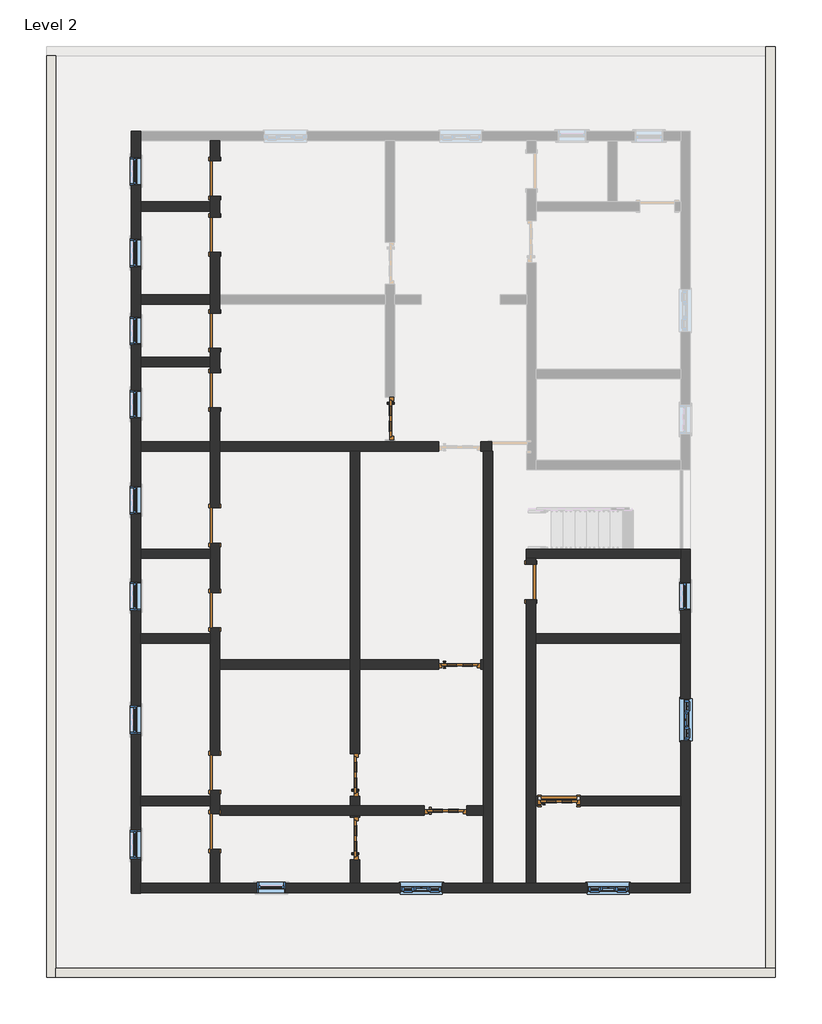
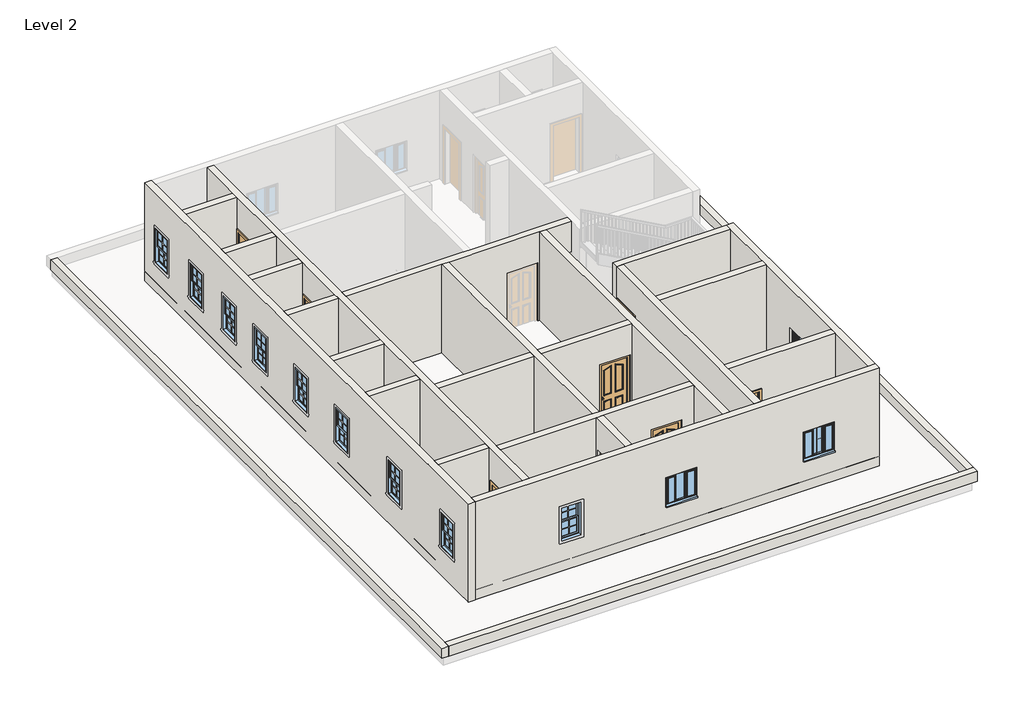
# One storey, part 1 of 3: 22 walls, 16 doors, 13 windows.
# Revit data of these elements (continued)
# Element 44 (IfcWindow, "Window-Double-Hung : 24\" x 42\"")
#   Mark = "28"
#   Window Inset = 0' - 0"
#   Interior Wall Closure = 0' - 1 1/2"
#   Frame Extension = 0' - 1 1/4"
#   Exterior Wall Closure = 0' - 0 1/2"
#   Interior Trim Visibility = yes
#   Indicator Visibility = yes
#   Exterior Trim Visibility = yes
#   Phase Created = New Construction
#   Materials on its faces: "Wood - Stained", "Glass", "Clad - White"
# Element 45 (IfcWindow, "Window-Double-Hung : 24\" x 42\"")
#   Mark = "29"
#   Window Inset = 0' - 0"
#   Interior Wall Closure = 0' - 1 1/2"
#   Frame Extension = 0' - 1 1/4"
#   Exterior Wall Closure = 0' - 0 1/2"
#   Interior Trim Visibility = yes
#   Indicator Visibility = yes
#   Exterior Trim Visibility = yes
#   Phase Created = New Construction
#   Materials on its faces: "Wood - Stained", "Glass", "Clad - White"
# Element 46 (IfcWindow, "Window-Double-Hung : 24\" x 42\"")
#   Mark = "30"
#   Window Inset = 0' - 0"
#   Interior Wall Closure = 0' - 1 1/2"
#   Frame Extension = 0' - 1 1/4"
#   Exterior Wall Closure = 0' - 0 1/2"
#   Interior Trim Visibility = yes
#   Indicator Visibility = yes
#   Exterior Trim Visibility = yes
#   Phase Created = New Construction
#   Materials on its faces: "Wood - Stained", "Glass", "Clad - White"
# Element 47 (IfcWindow, "Window-Double-Hung : 24\" x 42\"")
#   Mark = "31"
#   Window Inset = 0' - 0"
#   Interior Wall Closure = 0' - 1 1/2"
#   Frame Extension = 0' - 1 1/4"
#   Exterior Wall Closure = 0' - 0 1/2"
#   Interior Trim Visibility = yes
#   Indicator Visibility = yes
#   Exterior Trim Visibility = yes
#   Phase Created = New Construction
#   Materials on its faces: "Wood - Stained", "Glass", "Clad - White"
# Element 48 (IfcWindow, "Window-Double-Hung : 24\" x 42\"")
#   Mark = "32"
#   Window Inset = 0' - 0"
#   Interior Wall Closure = 0' - 1 1/2"
#   Frame Extension = 0' - 1 1/4"
#   Exterior Wall Closure = 0' - 0 1/2"
#   Interior Trim Visibility = yes
#   Indicator Visibility = yes
#   Exterior Trim Visibility = yes
#   Phase Created = New Construction
#   Materials on its faces: "Wood - Stained", "Glass", "Clad - White"
# Element 49 (IfcWindow, "Windows_Tpl_w-Glazing_Cross-Bars : 910x910mm")
#   Mark = "20"
#   Phase Created = New Construction
#   Materials on its faces: "Window Frame", "Glass"
# Element 50 (IfcWindow, "Windows_Tpl_w-Glazing_Cross-Bars : 910x910mm")
#   Mark = "37"
#   Phase Created = New Construction
#   Materials on its faces: "Window Frame", "Glass"
# Element 51 (IfcWindow, "Windows_Tpl_w-Glazing_Cross-Bars : 910x910mm")
#   Mark = "38"
#   Phase Created = New Construction
#   Materials on its faces: "Window Frame", "Glass"
# Materials
#   "Door - Glazing": colour RGB 0 0 255, transparency 0.75
#   "Door - Panel": class "Wood", colour RGB 210 159 95, transparency 0, Cost = 0
#   "Door - Frame/Mullion": class "Wood", colour RGB 212 179 113, transparency 0
#   "Door - Handle": colour RGB 246 240 166, transparency 0
#   "Door - Frame": colour RGB 118 70 51, transparency 0, Cost = 0
#   "Wood - Stained": class "Wood", colour RGB 224 178 126, transparency 0, Cost = 0
#   "Clad - White": class "Wood", colour RGB 242 242 238, transparency 0, Cost = 0
#   "Glass": class "Glass", colour RGB 0 128 192, transparency 0.75, Description = "Soda Lime Glass", Cost = 0
#   "Window Frame": colour RGB 249 249 249, transparency 0
#   "Default Wall": colour RGB 128 128 128, transparency 0, Cost = 0
#   "Tile, Porcelain, 4in": class "Generic", colour RGB 89 87 158, transparency 0, Description = "Porcelain tile, 4\", white", Cost = 0
